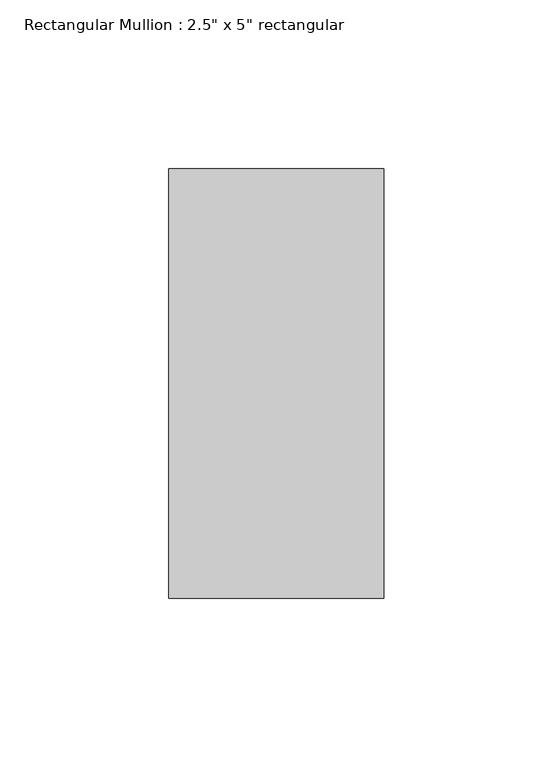
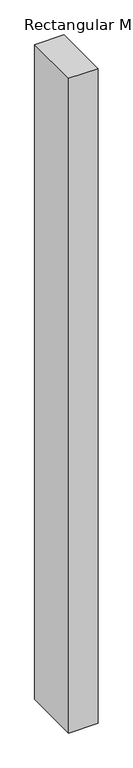
"""IFC4 building model written with IfcOpenShell, lengths in millimetres: member geometry."""

from ifc_helpers import new_model, si_unit, frame, origin, place, context, project, spatial, polyline, outline, extrude, source, transform, mapped, element, save


def member_466b835c(model_context):
    return source(origin(), model_context, "Body", "SweptSolid", [
        extrude(outline(polyline([(0.0, 63.5), (0.0, -63.5), (-63.5, -63.5), (-63.5, 63.5), (0.0, 63.5)])), frame((0.0, 0.0, -1494.7499719), z_axis=(0.0, 0.0, 1.0), x_axis=(1.0, 0.0, 0.0)), (0.0, 0.0, 1.0), 1494.7499719),
    ])


if __name__ == "__main__":
    model = new_model("IFC4")
    model_context = context("Model", 3, world=origin())
    ifc_project = project(units=[si_unit("LENGTHUNIT", "METRE", prefix="MILLI")], contexts=[model_context])
    site = spatial("IfcSite", under=ifc_project)
    building = spatial("IfcBuilding", under=site)
    placement = place(None, origin())
    member_shape = member_466b835c(model_context)
    element("IfcMember", 1, ObjectType="Rectangular Mullion : 2.5\" x 5\" rectangular", at=placement, inside=building, context=model_context, shape_type="MappedRepresentation", body=[
        mapped(member_shape, transform((0.0, 0.0, 0.0), x_axis=(1.0, 0.0, 0.0), y_axis=(0.0, 1.0, 0.0), z_axis=(0.0, 0.0, 1.0))),
    ])
    save(model, "model.ifc")

# Revit data of these elements
# Type "Rectangular Mullion : 2.5\" x 5\" rectangular"
#   built-in parameter 1007304 = 0.416667 (stored number, unit not read)
#   built-in parameter 1007301 = 0.104167 (stored number, unit not read)
#   built-in parameter 1007300 = 0.104167 (stored number, unit not read)
# Element 1 (IfcMember, "Rectangular Mullion : 2.5\" x 5\" rectangular")
#   Materials on its faces: "Aluminum"
# Materials
#   "Aluminum": class "Metal", colour RGB 247 247 247, transparency 0, Description = "Aluminum 6061", Cost = 0
